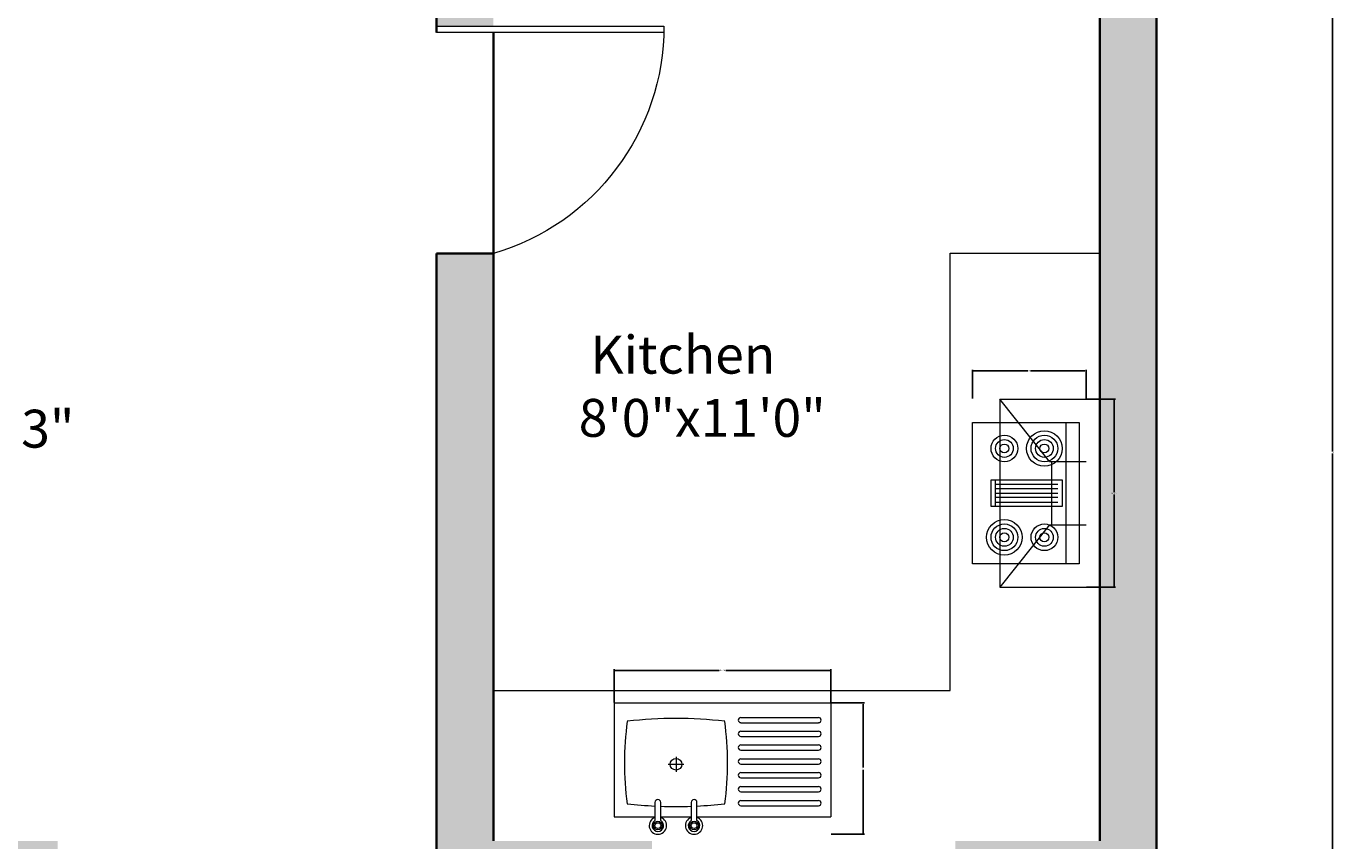
# Model space of a CAD drawing. Units: inches. Extents: x 1752 to 2227, y 6273 to 6884.
# Tile 4 of 6: x 2020 to 2227, y 6511 to 6640. Entities that reach past the tile are written whole.
import ezdxf

# ---------------------------------------------------------------- set-up
doc = ezdxf.new("R2010")
doc.units = ezdxf.units.IN
doc.header["$MEASUREMENT"] = 0
for name, color, linetype, lineweight in [('A-ANNO-DIMS', 2, 'Continuous', 18), ('A-AREA-IDEN', 7, 'Continuous', 18), ('A-DOOR', 3, 'Continuous', 20), ('A-EQPM', 8, 'Continuous', 18), ('A-FLOR-CASE', 8, 'Continuous', 20), ('A-FLOR-FIXT', 8, 'Continuous', 18), ('A-WALL', 7, 'Continuous', 35)]:
    doc.layers.add(name, color=color, linetype=linetype, lineweight=lineweight)
doc.layers.add('A-WALL-PATT', color=32, linetype='Continuous', lineweight=13, true_color=0xcd6928)
doc.styles.get("Standard").update_dxf_attribs({"font": 'arial.ttf'})
doc.dimstyles.get("Standard").update_dxf_attribs({"dimtxt": 0.18, "dimasz": 0.18, "dimexe": 0.18, "dimexo": 0.0625, "dimgap": 0.09, "dimtad": 0, "dimtih": 1, "dimtoh": 1, "dimdec": 4, "dimzin": 0, "dimdsep": 46, "dimtxsty": 'Standard', "dimcen": 0.09, "dimadec": 0, "dimazin": 0, "dimtfac": 1, "dimtdec": 4, "dimtofl": 0, "dimtmove": 0, "dimatfit": 3, "dimfxl": 1, "dimtolj": 1, "dimtzin": 0, "dimarcsym": 0})

# ---------------------------------------------------------------- blocks, each defined once
blk = doc.blocks.new('chimmne')
for p, q in [((17.89, 6.07), (-18.11, 6.07)), ((-18.11, 6.07), (-18.11, -10.43)), ((-6.16, -3.43), (-18.11, 6.07)), ((5.94, -3.43), (17.89, 6.07)), ((17.89, 6.07), (17.89, -10.43)), ((-6.16, -3.43), (-6.16, -10.43)), ((5.94, -3.82), (-6.16, -3.82)), ((5.94, -3.43), (5.94, -10.43))]:
    blk.add_line(p, q)
for points in [[(-13.61, -9.12), (-13.61, 11.28), (13.39, 11.28), (13.39, -9.12)], [(-2.66, -5.87), (-2.66, 7.73), (2.44, 7.73), (2.44, -5.87)]]:
    blk.add_lwpolyline(points, close=True)
for points in [[(-2.66, 6.88), (2.44, 6.88)], [(-1.81, 6.88), (-1.81, -5.02)], [(-0.96, -5.02), (-0.96, 6.88)], [(-0.11, 6.88), (-0.11, -5.02)], [(0.74, -5.02), (0.74, 6.88)], [(1.59, 6.88), (1.59, -5.02)], [(13.39, -6.57), (-13.61, -6.57)]]:
    blk.add_lwpolyline(points)
for centre, radius in [((-8.55, 5.18), 3.4), ((-8.55, 5.18), 2.55), ((8.44, 5.18), 2.55), ((-8.55, 5.18), 1.7), ((-8.55, 5.18), 0.85), ((8.44, 5.18), 1.7), ((8.44, 5.18), 0.85), ((-8.55, -2.47), 2.55), ((8.44, -2.47), 3.4), ((8.44, -2.47), 2.55), ((-8.55, -2.47), 1.7), ((-8.55, -2.47), 0.85), ((8.44, -2.47), 1.7), ((8.44, -2.47), 0.85)]:
    blk.add_circle(centre, radius)
blk = doc.blocks.new('A$C799204C7')
for p, q in [((0, 34.2), (17.99, 34.2)), ((0, 0), (0, 34.2)), ((17.99, 13.08), (17.99, 34.2)), ((2.32, 20.01), (2.32, 32.27)), ((3.13, 20.01), (3.13, 32.27)), ((4.48, 20.01), (4.48, 32.27)), ((5.29, 20.01), (5.29, 32.27)), ((6.64, 20.01), (6.64, 32.27)), ((7.45, 20.01), (7.45, 32.27)), ((8.85, 20.01), (8.85, 32.27)), ((9.66, 20.01), (9.66, 32.27)), ((11.01, 20.01), (11.01, 32.27)), ((11.82, 20.01), (11.82, 32.27)), ((13.22, 20.01), (13.22, 32.27)), ((14.03, 20.01), (14.03, 32.27)), ((15.42, 20.01), (15.42, 32.27)), ((16.24, 20.01), (16.24, 32.27)), ((18.59, 13.08), (15.71, 13.08)), ((9.73, 11), (9.73, 8.54)), ((15.71, 12.17), (18.59, 12.17)), ((17.99, 7.36), (17.99, 12.17)), ((8.52, 9.77), (10.9, 9.77)), ((18.59, 7.36), (15.71, 7.36)), ((15.71, 6.45), (18.59, 6.45)), ((17.99, 0), (17.99, 6.45)), ((0, 0), (17.99, 0))]:
    blk.add_line(p, q)
for centre, radius in [((19.38, 12.62), 0.684), ((19.38, 12.62), 0.456), ((9.7, 9.77), 0.916), ((19.38, 6.91), 0.684), ((19.38, 6.91), 0.456)]:
    blk.add_circle(centre, radius)
for centre, radius, start, end in [((2.72, 32.27), 0.407, 0, 180), ((4.88, 32.27), 0.407, 0, 180), ((7.05, 32.27), 0.407, 0, 180), ((9.25, 32.27), 0.407, 0, 180), ((11.42, 32.27), 0.407, 0, 180), ((13.62, 32.27), 0.407, 0, 180), ((15.83, 32.27), 0.407, 0, 180), ((2.72, 20.01), 0.407, 180, 0), ((4.88, 20.01), 0.407, 180, 0), ((7.05, 20.01), 0.407, 180, 0), ((9.25, 20.01), 0.407, 180, 0), ((11.42, 20.01), 0.407, 180, 0), ((13.62, 20.01), 0.407, 180, 0), ((15.83, 20.01), 0.407, 180, 0), ((67.33, 9.77), 64.88, 173.1952, 186.8048), ((9.53, -30.19), 48.1, 82.3437, 97.8966), ((-48.51, 9.77), 64.88, 2.9208, 6.8048), ((15.71, 12.62), 0.456, 90, 270), ((19.38, 12.62), 1.37, 199.6514, 160.3603), ((19.38, 12.62), 0.911, 210.3431, 149.7554), ((-48.51, 9.77), 64.88, 357.8723, 2.115), ((19.38, 6.91), 1.37, 199.6514, 160.3603), ((15.71, 6.91), 0.456, 90, 270), ((-48.51, 9.77), 64.88, 353.1952, 357.0665), ((19.38, 6.91), 0.911, 210.3431, 149.7554), ((9.53, 49.73), 48.1, 262.1034, 277.6563)]:
    blk.add_arc(centre, radius, start, end)
blk = doc.blocks.new('DOOR-SINGLE-36IN')
for p, q in [((35, 36), (35, 0)), ((36, 0), (36, 36)), ((36, 0), (35, 0))]:
    blk.add_line(p, q)
blk.add_arc((36, -1.5), 37.5, 90, 163.7398)
blk = doc.blocks.new('*D34')
at = {"layer": 'A-ANNO-DIMS', "color": 0, "lineweight": -2, "transparency": 16777216}
for p, q in [((2187.53, 6580.87), (2192.12, 6580.87)), ((2191.94, 6580.69), (2191.94, 6566.15)), ((2191.94, 6551.24), (2191.94, 6565.78)), ((2187.53, 6551.06), (2192.12, 6551.06))]:
    blk.add_line(p, q, dxfattribs=at)
at = {"layer": 'A-ANNO-DIMS', "color": 0, "transparency": 16777216}
for points in [[(2191.91, 6580.69), (2191.97, 6580.69), (2191.94, 6580.87)], [(2191.91, 6551.24), (2191.97, 6551.24), (2191.94, 6551.06)]]:
    blk.add_solid(points, dxfattribs=at)
at = {"layer": 'Defpoints', "color": 0, "transparency": 16777216}
for p in [(2187.47, 6580.87), (2191.94, 6580.87), (2187.47, 6551.06)]:
    blk.add_point(p, dxfattribs=at)
at = {"layer": 'A-ANNO-DIMS', "color": 0, "transparency": 16777216, "insert": (2191.94, 6565.96), "char_height": 0.18, "attachment_point": 5}
blk.add_mtext('\\A1;HOB 30', dxfattribs=at)
blk = doc.blocks.new('*D35')
at = {"layer": 'A-ANNO-DIMS', "color": 0, "lineweight": -2, "transparency": 16777216}
for p, q in [((2169.49, 6580.93), (2169.49, 6585.52)), ((2169.67, 6585.34), (2178.27, 6585.34)), ((2187.29, 6585.34), (2178.69, 6585.34)), ((2187.47, 6580.93), (2187.47, 6585.52))]:
    blk.add_line(p, q, dxfattribs=at)
at = {"layer": 'A-ANNO-DIMS', "color": 0, "transparency": 16777216}
for points in [[(2169.67, 6585.37), (2169.67, 6585.31), (2169.49, 6585.34)], [(2187.29, 6585.37), (2187.29, 6585.31), (2187.47, 6585.34)]]:
    blk.add_solid(points, dxfattribs=at)
at = {"layer": 'Defpoints', "color": 0, "transparency": 16777216}
for p in [(2169.49, 6585.34), (2169.49, 6580.87), (2187.47, 6580.87)]:
    blk.add_point(p, dxfattribs=at)
at = {"layer": 'A-ANNO-DIMS', "color": 0, "transparency": 16777216, "insert": (2178.48, 6585.34), "char_height": 0.18, "attachment_point": 5}
blk.add_mtext('\\A1;18', dxfattribs=at)
blk = doc.blocks.new('*D36')
at = {"layer": 'A-ANNO-DIMS', "color": 0, "lineweight": -2, "transparency": 16777216}
for p, q in [((2112.75, 6532.83), (2112.75, 6538.09)), ((2112.93, 6537.91), (2129.36, 6537.91)), ((2146.88, 6537.91), (2130.45, 6537.91)), ((2147.06, 6532.83), (2147.06, 6538.09))]:
    blk.add_line(p, q, dxfattribs=at)
at = {"layer": 'A-ANNO-DIMS', "color": 0, "transparency": 16777216}
for points in [[(2112.93, 6537.94), (2112.93, 6537.88), (2112.75, 6537.91)], [(2146.88, 6537.94), (2146.88, 6537.88), (2147.06, 6537.91)]]:
    blk.add_solid(points, dxfattribs=at)
at = {"layer": 'Defpoints', "color": 0, "transparency": 16777216}
for p in [(2147.06, 6537.91), (2112.75, 6532.76), (2147.06, 6532.76)]:
    blk.add_point(p, dxfattribs=at)
at = {"layer": 'A-ANNO-DIMS', "color": 0, "transparency": 16777216, "insert": (2129.9, 6537.91), "char_height": 0.18, "attachment_point": 5}
blk.add_mtext('\\A1;SINK 34', dxfattribs=at)
blk = doc.blocks.new('*D37')
at = {"layer": 'A-ANNO-DIMS', "color": 0, "lineweight": -2, "transparency": 16777216}
for p, q in [((2147.12, 6532.76), (2152.38, 6532.76)), ((2152.2, 6532.58), (2152.2, 6522.54)), ((2152.2, 6512.13), (2152.2, 6522.18)), ((2147.12, 6511.95), (2152.38, 6511.95))]:
    blk.add_line(p, q, dxfattribs=at)
at = {"layer": 'A-ANNO-DIMS', "color": 0, "transparency": 16777216}
for points in [[(2152.17, 6532.58), (2152.23, 6532.58), (2152.2, 6532.76)], [(2152.17, 6512.13), (2152.23, 6512.13), (2152.2, 6511.95)]]:
    blk.add_solid(points, dxfattribs=at)
at = {"layer": 'Defpoints', "color": 0, "transparency": 16777216}
for p in [(2147.06, 6532.76), (2147.06, 6511.95), (2152.2, 6511.95)]:
    blk.add_point(p, dxfattribs=at)
at = {"layer": 'A-ANNO-DIMS', "color": 0, "transparency": 16777216, "insert": (2152.2, 6522.36), "char_height": 0.18, "attachment_point": 5}
blk.add_mtext('\\A1;21', dxfattribs=at)
blk = doc.blocks.new('*D43')
at = {"layer": 'A-ANNO-DIMS', "color": 0, "lineweight": -2, "transparency": 16777216}
for p, q in [((2189.71, 6642.91), (2226.68, 6642.91)), ((2226.5, 6642.73), (2226.5, 6572.59)), ((2226.5, 6502.09), (2226.5, 6572.23)), ((2189.71, 6501.91), (2226.68, 6501.91))]:
    blk.add_line(p, q, dxfattribs=at)
at = {"layer": 'A-ANNO-DIMS', "color": 0, "transparency": 16777216}
for points in [[(2226.47, 6642.73), (2226.53, 6642.73), (2226.5, 6642.91)], [(2226.47, 6502.09), (2226.53, 6502.09), (2226.5, 6501.91)]]:
    blk.add_solid(points, dxfattribs=at)
at = {"layer": 'Defpoints', "color": 0, "transparency": 16777216}
for p in [(2189.65, 6642.91), (2226.5, 6642.91), (2189.65, 6501.91)]:
    blk.add_point(p, dxfattribs=at)
at = {"layer": 'A-ANNO-DIMS', "color": 0, "transparency": 16777216, "insert": (2226.5, 6572.41), "char_height": 0.18, "attachment_point": 5}
blk.add_mtext('\\A1;141', dxfattribs=at)

msp = doc.modelspace()

# ---------------------------------------------------------------- hatches: boundary and pattern name
at = {"layer": 'A-WALL-PATT'}
h = msp.add_hatch(color=256, dxfattribs=at)
h.dxf.hatch_style = 1
h.paths.add_polyline_path([(2198.6473, 6855.914), (1780.1473, 6855.914), (1780.1473, 6309.914), (1824.3861, 6309.914), (1824.3861, 6318.914), (1789.1473, 6318.914), (1789.1473, 6501.914), (1790.1473, 6501.914), (1790.1473, 6510.914), (1789.1473, 6510.914), (1789.1473, 6570.914), (1838.6473, 6570.914), (1838.6473, 6510.914), (1822.1473, 6510.914), (1822.1473, 6501.914), (1921.1473, 6501.914), (1921.1473, 6498.914), (1930.1473, 6498.914), (1930.1473, 6501.914), (1930.1473, 6510.914), (1847.6473, 6510.914), (1847.6473, 6585.039), (1838.6473, 6585.039), (1838.6473, 6575.414), (1789.1473, 6575.414), (1789.1473, 6705.914), (1795.2039, 6705.914), (1795.2039, 6714.914), (1789.1473, 6714.914), (1789.1473, 6846.914), (1984.1473, 6846.914), (1984.1473, 6714.914), (1977.8419, 6714.914), (1977.8419, 6705.914), (1984.1473, 6705.914), (1984.1473, 6651.914), (1977.6147, 6651.914), (1977.6147, 6642.914), (1996.1473, 6642.914), (1996.1473, 6651.914), (1993.1473, 6651.914), (1993.1473, 6846.914), (2125.1473, 6846.914), (2125.1473, 6840.4779), (2129.6473, 6840.4779), (2129.6473, 6846.914), (2189.6473, 6846.914), (2189.6473, 6798.914), (2162.6473, 6798.914), (2162.6473, 6794.414), (2189.6473, 6794.414), (2189.6473, 6710.414), (2175.6868, 6710.414), (2175.6868, 6705.914), (2189.6473, 6705.914), (2189.6473, 6651.914), (2164.6473, 6651.914), (2164.6473, 6642.914), (2189.6473, 6642.914), (2189.6473, 6510.914), (2166.7624, 6510.914), (2166.7624, 6501.914), (2189.6473, 6501.914), (2189.6473, 6318.914), (2173.9269, 6318.914), (2173.9269, 6309.914), (2198.6473, 6309.914)])
h.paths.add_polyline_path([(2023.6785, 6318.914), (1930.1473, 6318.914), (1930.1473, 6321.914), (1921.1473, 6321.914), (1921.1473, 6318.914), (1872.3861, 6318.914), (1872.3861, 6309.914), (2023.6785, 6309.914)], flags=17)
h.paths.add_polyline_path([(2092.7496, 6318.914), (2061.7431, 6318.914), (2061.7431, 6309.914), (2092.7496, 6309.914)], flags=0)
h.paths.add_polyline_path([(1947.0033, 6375.914), (1930.1473, 6375.914), (1930.1473, 6462.914), (1921.1473, 6462.914), (1921.1473, 6357.914), (1930.1473, 6357.914), (1930.1473, 6366.914), (1947.0033, 6366.914)], flags=17)
h.paths.add_polyline_path([(2024.6473, 6432.914), (2015.6473, 6432.914), (2015.6473, 6375.914), (1995.0033, 6375.914), (1995.0033, 6366.914), (2024.6473, 6366.914)], flags=17)
h.paths.add_polyline_path([(2030.6473, 6441.914), (2024.6473, 6441.914), (2024.6473, 6510.914), (2015.6473, 6510.914), (2015.6473, 6432.914), (2024.6473, 6432.914), (2030.6473, 6432.914)], flags=17)
h.paths.add_polyline_path([(2093.6473, 6501.914), (2118.7624, 6501.914), (2118.7624, 6510.914), (2093.6473, 6510.914), (2093.6473, 6603.914), (2084.6473, 6603.914), (2084.6473, 6441.914), (2078.6473, 6441.914), (2078.6473, 6432.914), (2093.6473, 6432.914)], flags=17)
h.paths.add_polyline_path([(2132.6473, 6651.914), (2129.6473, 6651.914), (2129.6473, 6705.914), (2139.6868, 6705.914), (2139.6868, 6710.414), (2129.6473, 6710.414), (2129.6473, 6794.414), (2130.6473, 6794.414), (2130.6473, 6798.914), (2129.6473, 6798.914), (2129.6473, 6804.4779), (2125.1473, 6804.4779), (2125.1473, 6651.914), (2032.1473, 6651.914), (2032.1473, 6642.914), (2084.6473, 6642.914), (2084.6473, 6639.914), (2093.6473, 6639.914), (2093.6473, 6642.914), (2132.6473, 6642.914)], flags=17)
h.paths.add_polyline_path([(1929.6147, 6651.914), (1924.1473, 6651.914), (1924.1473, 6705.914), (1941.8419, 6705.914), (1941.8419, 6714.914), (1911.8299, 6714.914), (1911.8299, 6705.914), (1919.6473, 6705.914), (1919.6473, 6651.914), (1847.6473, 6651.914), (1847.6473, 6662.4635), (1838.6473, 6662.4635), (1838.6473, 6621.039), (1847.6473, 6621.039), (1847.6473, 6642.914), (1929.6147, 6642.914)], flags=17)
h.paths.add_polyline_path([(1879.8299, 6714.914), (1831.2039, 6714.914), (1831.2039, 6705.914), (1838.6473, 6705.914), (1838.6473, 6698.4635), (1847.6473, 6698.4635), (1847.6473, 6705.914), (1879.8299, 6705.914)], flags=17)

# ---------------------------------------------------------------- linework, layer by layer
at = {"layer": 'A-FLOR-CASE'}
for p, q in [((2165.9563, 6534.6944), (2165.9563, 6603.9718)), ((2165.9563, 6603.9718), (2189.6473, 6603.9718)), ((2093.6473, 6534.6944), (2165.9563, 6534.6944))]:
    msp.add_line(p, q, dxfattribs=at)
at = {"layer": 'A-WALL'}
for p, q in [((2198.6473, 6855.914), (2198.6473, 6309.914)), ((2084.6473, 6642.914), (2084.6473, 6638.914)), ((2189.6473, 6642.914), (2189.6473, 6510.914)), ((2093.6473, 6638.914), (2093.6473, 6510.914)), ((2084.6473, 6603.914), (2093.6473, 6603.914)), ((2084.6473, 6603.914), (2084.6473, 6441.914))]:
    msp.add_line(p, q, dxfattribs=at)

# ---------------------------------------------------------------- block references
at = {"layer": 'A-DOOR', "extrusion": (0, 0, -1), "zscale": -1, "rotation": 90.0000000000043}
msp.add_blockref('DOOR-SINGLE-36IN', (-2084.6473, 6603.9141), dxfattribs=at)
at = {"layer": 'A-EQPM', "xscale": 0.8280321260258986, "yscale": 0.8280321260258986, "zscale": 0.8280321260258986, "rotation": 90}
msp.add_blockref('chimmne', (2178.8292, 6566.0572), dxfattribs=at)
at = {"layer": 'A-FLOR-FIXT', "xscale": 1.0032, "yscale": 1.0032, "zscale": 1.0032, "rotation": 270}
msp.add_blockref('A$C799204C7', (2112.7482, 6532.765), dxfattribs=at)

# ---------------------------------------------------------------- texts
at = {"layer": 'A-AREA-IDEN', "char_height": 6, "attachment_point": 1}
for s, width, insert in [(' Kitchen\\P8\'0"x11\'0"', 45.442011, (2107.1454, 6590.893)), ('      Hall\\P20\'3"x11\'3"', 75.076462, (1983.6553, 6589.178))]:
    msp.add_mtext_dynamic_manual_height_columns(s, width=width, gutter_width=30, heights=[0], dxfattribs=dict(at, insert=insert))

# ---------------------------------------------------------------- dimensions: what is measured, and where the dimension line sits
at = {"layer": 'A-ANNO-DIMS'}
for base, p1, p2, angle, picture, middle in [((2226.4973, 6642.914), (2189.6473, 6501.914), (2189.6473, 6642.914), 90, '*D43', (2226.4973, 6572.414)), ((2169.4919, 6585.3402), (2187.4654, 6580.8689), (2169.4919, 6580.8689), 180, '*D35', (2178.4787, 6585.3402)), ((2152.204, 6511.9509), (2147.0576, 6532.765), (2147.0576, 6511.9509), 270, '*D37', (2152.204, 6522.3579))]:
    dim = msp.add_linear_dim(base=base, p1=p1, p2=p2, angle=angle, dimstyle='Standard', override={"dimdec": 0, "dimlfac": 1, "dimrnd": 0, "dimzin": 0, "dimdsep": 46, "dimlunit": 2}, dxfattribs=at)
    dim.commit()
    dim.dimension.update_dxf_attribs({"geometry": picture, "text_midpoint": middle})
dim = msp.add_linear_dim(base=(2191.9368, 6580.8689), p1=(2187.4654, 6551.0597), p2=(2187.4654, 6580.8689), angle=90, text='HOB <>', dimstyle='Standard', override={"dimdec": 0, "dimlfac": 1, "dimrnd": 0, "dimzin": 0, "dimdsep": 46, "dimlunit": 2}, dxfattribs=at)
dim.commit()
dim.dimension.update_dxf_attribs({"geometry": '*D34', "text_midpoint": (2191.9368, 6565.9643)})
dim = msp.add_linear_dim(base=(2147.0576, 6537.9114), p1=(2112.7482, 6532.765), p2=(2147.0576, 6532.765), text='SINK <>', dimstyle='Standard', override={"dimdec": 0, "dimlfac": 1, "dimrnd": 0, "dimzin": 0, "dimdsep": 46, "dimlunit": 2}, dxfattribs=at)
dim.commit()
dim.dimension.update_dxf_attribs({"geometry": '*D36', "text_midpoint": (2129.9029, 6537.9114)})

doc.saveas('drawing.dxf')
